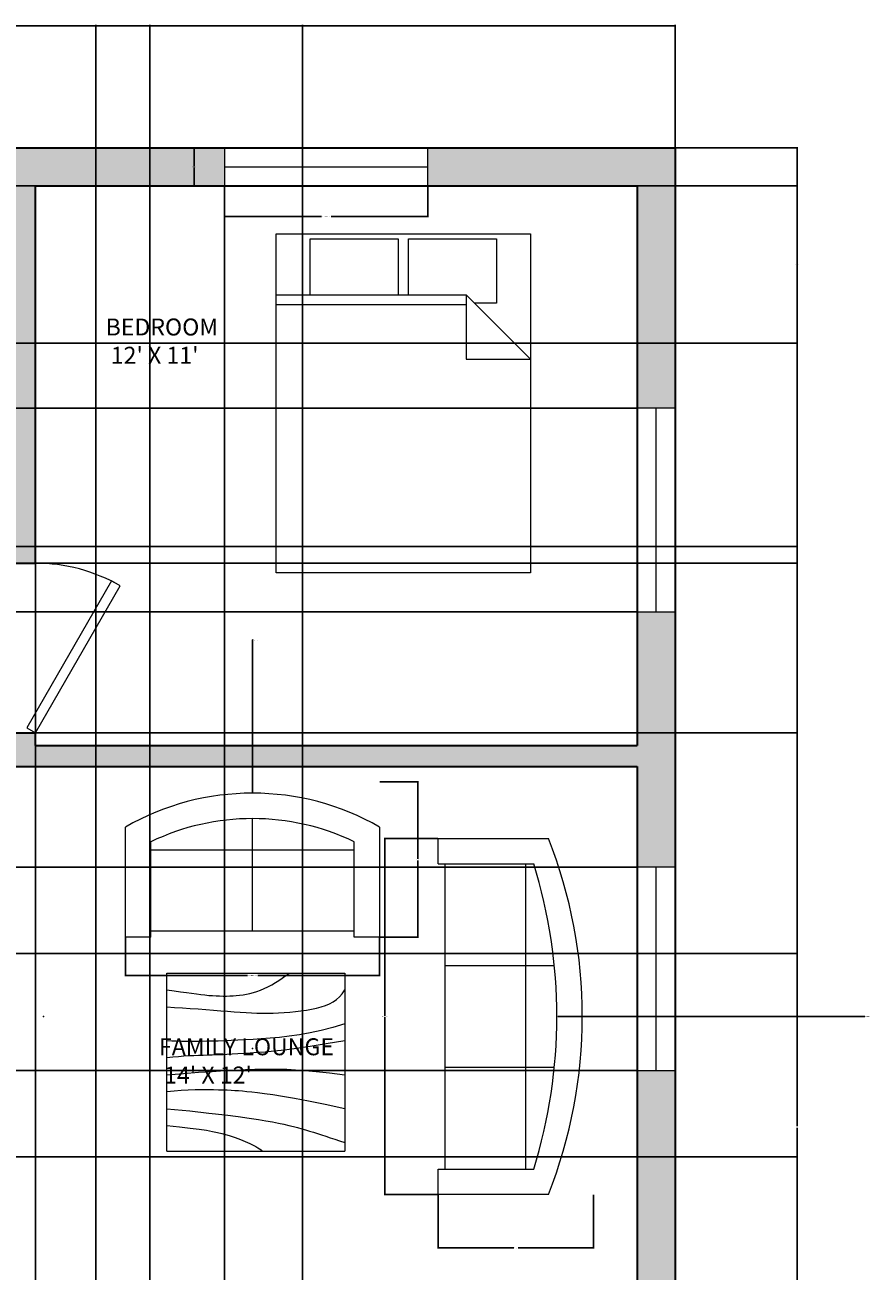
# Model space of a CAD drawing. Units: inches. Extents: x -28 to 649, y -11 to 509.
# Tile 7 of 7: x 450 to 649, y 215 to 509. Entities that reach past the tile are written whole.
import ezdxf

# ---------------------------------------------------------------- set-up
doc = ezdxf.new("R2010")
doc.units = ezdxf.units.IN
doc.header["$MEASUREMENT"] = 0
for name, color, linetype, lineweight in [('A-ANNO-DIMS', 2, 'Continuous', 18), ('A-AREA-IDEN', 18, 'Continuous', 18), ('A-WALL', 7, 'Continuous', 35), ('A-WALL-PATT', 251, 'Continuous', 13), ('doors', 40, 'Continuous', 20), ('furniture', 220, 'Continuous', 18), ('window', 30, 'Continuous', 18)]:
    doc.layers.add(name, color=color, linetype=linetype, lineweight=lineweight)
doc.styles.get("Standard").update_dxf_attribs({"font": 'arial.ttf'})
doc.dimstyles.get("Standard").update_dxf_attribs({"dimtxt": 0.18, "dimasz": 0.18, "dimexe": 0.18, "dimexo": 0.0625, "dimgap": 0.09, "dimtad": 0, "dimtih": 1, "dimtoh": 1, "dimdec": 4, "dimzin": 0, "dimdsep": 46, "dimtxsty": 'Standard', "dimcen": 0.09, "dimadec": 0, "dimazin": 0, "dimtfac": 1, "dimtdec": 4, "dimtofl": 0, "dimtmove": 0, "dimatfit": 3, "dimfxl": 1, "dimtolj": 1, "dimtzin": 0, "dimarcsym": 0})

# ---------------------------------------------------------------- blocks, each defined once
blk = doc.blocks.new('*U10')
for p, q in [((0, 0), (0, 100)), ((750, 0), (750, 100))]:
    blk.add_line(p, q)
blk.add_lwpolyline([(0, 0), (649.5, -375), (671.4, -337.1), (21.9, 37.9)], close=True)
blk.add_arc((0, 0), 750, 330, 0)
blk = doc.blocks.new('Sofa - Roundback 7 ft.')
for p, q in [((-12.00002, -32.4421), (-12.00003, -6.5971)), ((11.99997, -32.4421), (11.99998, -6.5971)), ((-36.000027, -34), (-36.000027, -11.4696)), ((35.99998, -34), (35.99998, -11.4696)), ((-35.999844, -13.3819), (35.9998, -13.3819)), ((-36.000027, -32.4421), (35.99998, -32.4421))]:
    blk.add_line(p, q)
for points in [[(-36.000027, -34), (-42.000027, -34), (-42.000027, -8)], [(41.99998, -8), (41.99998, -34), (35.99998, -34)]]:
    blk.add_lwpolyline(points)
for centre, radius, start, end in [((0, -114.25), 114.25, 68.43141, 111.5686), ((-0.00001, -127.1968), 121.1968, 72.72033, 107.2797)]:
    blk.add_arc(centre, radius, start, end)
blk = doc.blocks.new('Sofa - Roundback Loveseat 5 ft.')
for p, q in [((0, -32.44198), (0, -5.99998)), ((-24, -33.99998), (-24, -11.46958)), ((24.00004, -33.99998), (24.00004, -11.46958)), ((-23.9998, -13.38178), (23.99986, -13.38178)), ((-24, -32.44198), (24.00004, -32.44198))]:
    blk.add_line(p, q)
for points in [[(-24, -33.99998), (-30, -33.99998), (-30, -7.99998)], [(30.00004, -7.99998), (30.00004, -33.99998), (24.00004, -33.99998)]]:
    blk.add_lwpolyline(points)
for centre, radius, start, end in [((0, -60.24998), 60.24998, 60.13715, 119.8628), ((0, -61.38438), 55.38444, 64.32083, 115.6792)]:
    blk.add_arc(centre, radius, start, end)
blk = doc.blocks.new('Bed - Queen')
for p, q in [((0, -80.00003), (0, 0)), ((0, 0), (59.99999, 0)), ((59.99999, 0), (59.99999, -80.00003)), ((7.99999, -1.2), (28.79998, -1.2)), ((7.99999, -14.4), (7.99999, -1.2)), ((28.79998, -1.2), (28.79998, -14.4)), ((31.19999, -1.2), (51.99999, -1.2)), ((31.19999, -14.4), (31.19999, -1.2)), ((51.99999, -1.2), (51.99999, -16.4)), ((0, -14.4), (44.8, -14.4)), ((59.99999, -29.6), (44.8, -14.4)), ((44.8, -14.4), (44.8, -29.6)), ((44.8, -16.8), (0, -16.8)), ((51.99999, -16.4), (46.79936, -16.4)), ((44.8, -29.6), (59.99999, -29.6)), ((59.99999, -80.00003), (0, -80.00003))]:
    blk.add_line(p, q)
blk = doc.blocks.new('Table - Square Woodgrain 42 x 42 in.')
blk.add_line((0, -42), (42, -42))
for points in [[(0, -4), (1.704, -4.2172), (3.2358, -4.4188), (4.615, -4.604), (5.8615, -4.7721), (6.9951, -4.9224), (8.0357, -5.0541), (9.0031, -5.1667), (9.9171, -5.2594), (10.7951, -5.3316), (11.6445, -5.3836), (12.4702, -5.4157), (13.277, -5.4283), (14.0698, -5.4217), (14.8535, -5.3964), (15.6331, -5.3526), (16.4133, -5.2908), (17.1986, -5.2103), (17.9913, -5.1062), (18.793, -4.9727), (19.6056, -4.8038), (20.4307, -4.5937), (21.2701, -4.3365), (22.1256, -4.0262), (22.9989, -3.6571), (23.888, -3.2272), (24.7756, -2.7516), (25.6408, -2.2491), (26.4624, -1.7387), (27.2195, -1.2395), (27.891, -0.7703), (28.456, -0.3501), (28.8934, 0.002)], [(0, -42), (0, 0), (42, 0), (42, -42)], [(0, -8), (1.8203, -8.1001), (3.6741, -8.2149), (5.5411, -8.3408), (7.4011, -8.4741), (9.2339, -8.6112), (11.0193, -8.7484), (12.7371, -8.8821), (14.3671, -9.0086), (15.8954, -9.1246), (17.3337, -9.2278), (18.6997, -9.3159), (20.0116, -9.387), (21.2871, -9.4389), (22.5442, -9.4696), (23.8008, -9.477), (25.0749, -9.459), (26.3791, -9.4137), (27.7049, -9.3403), (29.0383, -9.2382), (30.3655, -9.1068), (31.6728, -8.9455), (32.9461, -8.7535), (34.1717, -8.5304), (35.3358, -8.2756), (36.4268, -7.9863), (37.443, -7.6521), (38.3849, -7.2603), (39.253, -6.7986), (40.048, -6.2542), (40.7705, -5.6147), (41.421, -4.8674), (42, -4)], [(42, -12), (39.1784, -12.8621), (36.4519, -13.5654), (33.8246, -14.1294), (31.3004, -14.5731), (28.8832, -14.9161), (26.577, -15.1775), (24.3858, -15.3768), (22.3136, -15.5332), (20.3622, -15.6632), (18.5254, -15.7718), (16.7947, -15.8612), (15.1618, -15.9338), (13.6183, -15.9916), (12.1558, -16.0369), (10.7659, -16.0718), (9.4403, -16.0987), (8.1703, -16.1191), (6.9461, -16.1325), (5.7577, -16.1377), (4.595, -16.1335), (3.4479, -16.1188), (2.3064, -16.0924), (1.1604, -16.0532), (0, -16)], [(42, -16), (37.6529, -16.7365), (33.8802, -17.329), (30.6179, -17.7961), (27.8015, -18.1561), (25.3668, -18.4275), (23.2497, -18.6288), (21.3859, -18.7785), (19.7111, -18.8949), (18.1693, -18.9939), (16.7375, -19.0795), (15.401, -19.1534), (14.1449, -19.217), (12.9544, -19.2717), (11.8148, -19.3191), (10.7113, -19.3606), (9.6291, -19.3976), (8.5534, -19.4323), (7.47, -19.4689), (6.3643, -19.5122), (5.222, -19.5672), (4.0288, -19.6386), (2.7703, -19.7313), (1.4321, -19.8501), (0, -20)], [(0, -24), (3.9243, -23.6805), (7.4766, -23.4138), (10.6891, -23.1954), (13.5943, -23.0205), (16.2247, -22.8847), (18.6125, -22.7832), (20.7903, -22.7116), (22.7903, -22.6651), (24.6563, -22.642), (26.4764, -22.6507), (28.35, -22.7024), (30.3766, -22.8084), (32.6555, -22.98), (35.2861, -23.2283), (38.3678, -23.5645), (42, -24)], [(42, -32), (37.392, -31.017), (33.4585, -30.2231), (30.1291, -29.5949), (27.3334, -29.109), (25.0009, -28.742), (23.0612, -28.4707), (21.4439, -28.2716), (20.0786, -28.1215), (18.8998, -28.0002), (17.8609, -27.9014), (16.9206, -27.8219), (16.0371, -27.7588), (15.1691, -27.709), (14.2748, -27.6693), (13.3128, -27.6368), (12.2415, -27.6083), (11.0295, -27.5824), (9.6867, -27.5643), (8.233, -27.5608), (6.6884, -27.5787), (5.0728, -27.6248), (3.4062, -27.7058), (1.7086, -27.8286), (0, -28)], [(0, -32), (5.4026, -32.5358), (9.9494, -33.019), (13.7424, -33.4553), (16.8834, -33.8505), (19.4743, -34.2106), (21.6171, -34.5413), (23.4136, -34.8486), (24.9657, -35.1382), (26.3614, -35.4156), (27.6332, -35.6841), (28.7995, -35.9467), (29.8788, -36.2064), (30.8897, -36.4661), (31.8507, -36.7288), (32.7802, -36.9973), (33.6968, -37.2747), (34.6175, -37.5635), (35.5531, -37.8651), (36.5128, -38.1805), (37.506, -38.5108), (38.5421, -38.8568), (39.6302, -39.2197), (40.7797, -39.6004), (42, -40)], [(0, -36), (3.0098, -36.2857), (5.5354, -36.5643), (7.6368, -36.8359), (9.374, -37.1009), (10.807, -37.3597), (11.9957, -37.6126), (13.0002, -37.8599), (13.8804, -38.102), (14.6874, -38.3393), (15.4365, -38.5729), (16.1338, -38.8041), (16.7858, -39.0341), (17.3987, -39.264), (17.9787, -39.4952), (18.5322, -39.7288), (19.0655, -39.9662), (19.5832, -40.2081), (20.0842, -40.4544), (20.5657, -40.7046), (21.0249, -40.9581), (21.459, -41.2144), (21.8653, -41.4731), (22.2409, -41.7335), (22.5831, -41.9951)]]:
    blk.add_lwpolyline(points)
blk = doc.blocks.new('WIN-48x9')
for p, q in [((9, 48), (0, 48)), ((0, 48), (0, 0)), ((4.5, 0), (4.5, 48)), ((9, 0), (9, 48)), ((0, 0), (9, 0)), ((0, 0), (4.5, 0))]:
    blk.add_line(p, q)
blk = doc.blocks.new('*D14')
at = {"layer": 'A-ANNO-DIMS', "color": 0, "lineweight": -2, "transparency": 16777216}
for p, q in [((497.1, 470.88), (497.1, 463.56)), ((545.1, 470.88), (545.1, 463.56)), ((497.28, 463.74), (519.98, 463.74)), ((544.92, 463.74), (522.21, 463.74))]:
    blk.add_line(p, q, dxfattribs=at)
at = {"layer": 'A-ANNO-DIMS', "color": 0, "transparency": 16777216}
for points in [[(497.28, 463.77), (497.28, 463.71), (497.1, 463.74)], [(544.92, 463.77), (544.92, 463.71), (545.1, 463.74)]]:
    blk.add_solid(points, dxfattribs=at)
at = {"layer": 'Defpoints', "color": 0, "transparency": 16777216}
for p in [(497.1, 470.94), (545.1, 470.94), (545.1, 463.74)]:
    blk.add_point(p, dxfattribs=at)
at = {"layer": 'A-ANNO-DIMS', "color": 0, "transparency": 16777216, "insert": (521.1, 463.74), "char_height": 0.18, "attachment_point": 5}
blk.add_mtext('\\A1;WINDOW 48 TYP.', dxfattribs=at)
blk = doc.blocks.new('*D15')
at = {"layer": 'A-ANNO-DIMS', "color": 0, "lineweight": -2, "transparency": 16777216}
for p, q in [((497.03, 479.94), (489.72, 479.94)), ((489.9, 479.76), (489.9, 475.62)), ((489.9, 471.12), (489.9, 475.26)), ((497.03, 470.94), (489.72, 470.94))]:
    blk.add_line(p, q, dxfattribs=at)
at = {"layer": 'A-ANNO-DIMS', "color": 0, "transparency": 16777216}
for points in [[(489.87, 479.76), (489.93, 479.76), (489.9, 479.94)], [(489.87, 471.12), (489.93, 471.12), (489.9, 470.94)]]:
    blk.add_solid(points, dxfattribs=at)
at = {"layer": 'Defpoints', "color": 0, "transparency": 16777216}
for p in [(497.1, 479.94), (489.9, 470.94), (497.1, 470.94)]:
    blk.add_point(p, dxfattribs=at)
at = {"layer": 'A-ANNO-DIMS', "color": 0, "transparency": 16777216, "insert": (489.9, 475.44), "char_height": 0.18, "attachment_point": 5}
blk.add_mtext('\\A1;9 TYP.', dxfattribs=at)
blk = doc.blocks.new('*D24')
at = {"layer": 'A-ANNO-DIMS', "color": 0, "lineweight": -2, "transparency": 16777216}
for p, q in [((547.46, 317.01), (534.75, 317.01)), ((534.93, 316.83), (534.93, 275.19)), ((534.93, 233.19), (534.93, 274.83)), ((547.46, 233.01), (534.75, 233.01))]:
    blk.add_line(p, q, dxfattribs=at)
at = {"layer": 'A-ANNO-DIMS', "color": 0, "transparency": 16777216}
for points in [[(534.9, 316.83), (534.96, 316.83), (534.93, 317.01)], [(534.9, 233.19), (534.96, 233.19), (534.93, 233.01)]]:
    blk.add_solid(points, dxfattribs=at)
at = {"layer": 'Defpoints', "color": 0, "transparency": 16777216}
for p in [(547.53, 317.01), (534.93, 233.01), (547.53, 233.01)]:
    blk.add_point(p, dxfattribs=at)
at = {"layer": 'A-ANNO-DIMS', "color": 0, "transparency": 16777216, "insert": (534.93, 275.01), "char_height": 0.18, "attachment_point": 5}
blk.add_mtext('\\A1;SOFA 84 TYP.', dxfattribs=at)
blk = doc.blocks.new('*D25')
at = {"layer": 'A-ANNO-DIMS', "color": 0, "lineweight": -2, "transparency": 16777216}
for p, q in [((547.53, 232.95), (547.53, 220.23)), ((584.19, 232.95), (584.19, 220.23)), ((547.71, 220.41), (565.33, 220.41)), ((584.01, 220.41), (566.39, 220.41))]:
    blk.add_line(p, q, dxfattribs=at)
at = {"layer": 'A-ANNO-DIMS', "color": 0, "transparency": 16777216}
for points in [[(547.71, 220.44), (547.71, 220.38), (547.53, 220.41)], [(584.01, 220.44), (584.01, 220.38), (584.19, 220.41)]]:
    blk.add_solid(points, dxfattribs=at)
at = {"layer": 'Defpoints', "color": 0, "transparency": 16777216}
for p in [(547.53, 233.01), (584.19, 233.01), (584.19, 220.41)]:
    blk.add_point(p, dxfattribs=at)
at = {"layer": 'A-ANNO-DIMS', "color": 0, "transparency": 16777216, "insert": (565.86, 220.41), "char_height": 0.18, "attachment_point": 5}
blk.add_mtext('\\A1;37 TYP.', dxfattribs=at)
blk = doc.blocks.new('*D26')
at = {"layer": 'A-ANNO-DIMS', "color": 0, "lineweight": -2, "transparency": 16777216}
for p, q in [((473.68, 293.62), (473.68, 284.5)), ((533.68, 293.62), (533.68, 284.5)), ((473.86, 284.68), (502.46, 284.68)), ((533.5, 284.68), (504.9, 284.68))]:
    blk.add_line(p, q, dxfattribs=at)
at = {"layer": 'A-ANNO-DIMS', "color": 0, "transparency": 16777216}
for points in [[(473.86, 284.71), (473.86, 284.65), (473.68, 284.68)], [(533.5, 284.71), (533.5, 284.65), (533.68, 284.68)]]:
    blk.add_solid(points, dxfattribs=at)
at = {"layer": 'Defpoints', "color": 0, "transparency": 16777216}
for p in [(473.68, 293.68), (533.68, 293.68), (533.68, 284.68)]:
    blk.add_point(p, dxfattribs=at)
at = {"layer": 'A-ANNO-DIMS', "color": 0, "transparency": 16777216, "insert": (503.68, 284.68), "char_height": 0.18, "attachment_point": 5}
blk.add_mtext('\\A1;LOVESEAT 60 TYP.', dxfattribs=at)
blk = doc.blocks.new('*D27')
at = {"layer": 'A-ANNO-DIMS', "color": 0, "lineweight": -2, "transparency": 16777216}
for p, q in [((533.74, 330.35), (542.86, 330.35)), ((542.68, 330.17), (542.68, 312.2)), ((542.68, 293.86), (542.68, 311.83)), ((533.74, 293.68), (542.86, 293.68))]:
    blk.add_line(p, q, dxfattribs=at)
at = {"layer": 'A-ANNO-DIMS', "color": 0, "transparency": 16777216}
for points in [[(542.65, 330.17), (542.71, 330.17), (542.68, 330.35)], [(542.65, 293.86), (542.71, 293.86), (542.68, 293.68)]]:
    blk.add_solid(points, dxfattribs=at)
at = {"layer": 'Defpoints', "color": 0, "transparency": 16777216}
for p in [(533.68, 330.35), (542.68, 330.35), (533.68, 293.68)]:
    blk.add_point(p, dxfattribs=at)
at = {"layer": 'A-ANNO-DIMS', "color": 0, "transparency": 16777216, "insert": (542.68, 312.02), "char_height": 0.18, "attachment_point": 5}
blk.add_mtext('\\A1;37 TYP.', dxfattribs=at)
blk = doc.blocks.new('*D30')
at = {"layer": 'A-ANNO-DIMS', "color": 0, "lineweight": -2, "transparency": 16777216}
for p, q in [((27.45, 480), (27.45, 508.92)), ((27.63, 508.74), (315.16, 508.74)), ((603.27, 508.74), (315.74, 508.74)), ((603.45, 480), (603.45, 508.92))]:
    blk.add_line(p, q, dxfattribs=at)
at = {"layer": 'A-ANNO-DIMS', "color": 0, "transparency": 16777216}
for points in [[(27.63, 508.77), (27.63, 508.71), (27.45, 508.74)], [(603.27, 508.77), (603.27, 508.71), (603.45, 508.74)]]:
    blk.add_solid(points, dxfattribs=at)
at = {"layer": 'Defpoints', "color": 0, "transparency": 16777216}
for p in [(603.45, 508.74), (27.45, 479.94), (603.45, 479.94)]:
    blk.add_point(p, dxfattribs=at)
at = {"layer": 'A-ANNO-DIMS', "color": 0, "transparency": 16777216, "insert": (315.45, 508.74), "char_height": 0.18, "attachment_point": 5}
blk.add_mtext('\\A1;576', dxfattribs=at)
blk = doc.blocks.new('*D31')
at = {"layer": 'A-ANNO-DIMS', "color": 0, "lineweight": -2, "transparency": 16777216}
for p, q in [((603.51, 479.94), (632.43, 479.94)), ((632.25, 479.76), (632.25, 249.12)), ((632.25, 18.12), (632.25, 248.76)), ((346.51, 17.94), (632.43, 17.94))]:
    blk.add_line(p, q, dxfattribs=at)
at = {"layer": 'A-ANNO-DIMS', "color": 0, "transparency": 16777216}
for points in [[(632.22, 479.76), (632.28, 479.76), (632.25, 479.94)], [(632.22, 18.12), (632.28, 18.12), (632.25, 17.94)]]:
    blk.add_solid(points, dxfattribs=at)
at = {"layer": 'Defpoints', "color": 0, "transparency": 16777216}
for p in [(603.45, 479.94), (632.25, 479.94), (346.45, 17.94)]:
    blk.add_point(p, dxfattribs=at)
at = {"layer": 'A-ANNO-DIMS', "color": 0, "transparency": 16777216, "insert": (632.25, 248.94), "char_height": 0.18, "attachment_point": 5}
blk.add_mtext('\\A1;462', dxfattribs=at)
blk = doc.blocks.new('*D48')
at = {"layer": 'A-ANNO-DIMS', "color": 0, "lineweight": -2, "transparency": 16777216}
for p, q in [((452.45, 470.88), (452.45, -11.04)), ((497.1, 470.88), (497.1, -11.04)), ((452.63, -10.86), (474.38, -10.86)), ((496.92, -10.86), (475.17, -10.86))]:
    blk.add_line(p, q, dxfattribs=at)
at = {"layer": 'A-ANNO-DIMS', "color": 0, "transparency": 16777216}
for points in [[(452.63, -10.83), (452.63, -10.89), (452.45, -10.86)], [(496.92, -10.83), (496.92, -10.89), (497.1, -10.86)]]:
    blk.add_solid(points, dxfattribs=at)
at = {"layer": 'Defpoints', "color": 0, "transparency": 16777216}
for p in [(452.45, 470.94), (497.1, 470.94), (497.1, -10.86)]:
    blk.add_point(p, dxfattribs=at)
at = {"layer": 'A-ANNO-DIMS', "color": 0, "transparency": 16777216, "insert": (474.77, -10.86), "char_height": 0.18, "attachment_point": 5}
blk.add_mtext('\\A1;44.65', dxfattribs=at)
blk = doc.blocks.new('*D49')
at = {"layer": 'A-ANNO-DIMS', "color": 0, "lineweight": -2, "transparency": 16777216}
for p, q in [((36.51, 470.94), (632.43, 470.94)), ((632.25, 470.76), (632.25, 452.59)), ((632.25, 434.06), (632.25, 452.23)), ((36.51, 433.88), (632.43, 433.88))]:
    blk.add_line(p, q, dxfattribs=at)
at = {"layer": 'A-ANNO-DIMS', "color": 0, "transparency": 16777216}
for points in [[(632.22, 470.76), (632.28, 470.76), (632.25, 470.94)], [(632.22, 434.06), (632.28, 434.06), (632.25, 433.88)]]:
    blk.add_solid(points, dxfattribs=at)
at = {"layer": 'Defpoints', "color": 0, "transparency": 16777216}
for p in [(36.45, 470.94), (36.45, 433.88), (632.25, 433.88)]:
    blk.add_point(p, dxfattribs=at)
at = {"layer": 'A-ANNO-DIMS', "color": 0, "transparency": 16777216, "insert": (632.25, 452.41), "char_height": 0.18, "attachment_point": 5}
blk.add_mtext('\\A1;37.055', dxfattribs=at)
blk = doc.blocks.new('*D50')
at = {"layer": 'A-ANNO-DIMS', "color": 0, "lineweight": -2, "transparency": 16777216}
for p, q in [((594.39, 470.94), (-1.53, 470.94)), ((-1.35, 470.76), (-1.35, 444.89)), ((-1.35, 418.66), (-1.35, 444.53)), ((594.39, 418.48), (-1.53, 418.48))]:
    blk.add_line(p, q, dxfattribs=at)
at = {"layer": 'A-ANNO-DIMS', "color": 0, "transparency": 16777216}
for points in [[(-1.38, 470.76), (-1.32, 470.76), (-1.35, 470.94)], [(-1.38, 418.66), (-1.32, 418.66), (-1.35, 418.48)]]:
    blk.add_solid(points, dxfattribs=at)
at = {"layer": 'Defpoints', "color": 0, "transparency": 16777216}
for p in [(594.45, 470.94), (-1.35, 418.48), (594.45, 418.48)]:
    blk.add_point(p, dxfattribs=at)
at = {"layer": 'A-ANNO-DIMS', "color": 0, "transparency": 16777216, "insert": (-1.35, 444.71), "char_height": 0.18, "attachment_point": 5}
blk.add_mtext('\\A1;52.46', dxfattribs=at)
blk = doc.blocks.new('*D51')
at = {"layer": 'A-ANNO-DIMS', "color": 0, "lineweight": -2, "transparency": 16777216}
for p, q in [((594.39, 370.48), (-1.53, 370.48)), ((-1.35, 370.3), (-1.35, 340.55)), ((-1.35, 310.43), (-1.35, 340.19)), ((594.39, 310.25), (-1.53, 310.25))]:
    blk.add_line(p, q, dxfattribs=at)
at = {"layer": 'A-ANNO-DIMS', "color": 0, "transparency": 16777216}
for points in [[(-1.38, 370.3), (-1.32, 370.3), (-1.35, 370.48)], [(-1.38, 310.43), (-1.32, 310.43), (-1.35, 310.25)]]:
    blk.add_solid(points, dxfattribs=at)
at = {"layer": 'Defpoints', "color": 0, "transparency": 16777216}
for p in [(-1.35, 370.48), (594.45, 370.48), (594.45, 310.25)]:
    blk.add_point(p, dxfattribs=at)
at = {"layer": 'A-ANNO-DIMS', "color": 0, "transparency": 16777216, "insert": (-1.35, 340.37), "char_height": 0.18, "attachment_point": 5}
blk.add_mtext('\\A1;60.23', dxfattribs=at)
blk = doc.blocks.new('*D52')
at = {"layer": 'A-ANNO-DIMS', "color": 0, "lineweight": -2, "transparency": 16777216}
for p, q in [((594.39, 262.25), (-1.53, 262.25)), ((-1.35, 262.07), (-1.35, 206.61)), ((-1.35, 150.79), (-1.35, 206.25)), ((594.39, 150.61), (-1.53, 150.61))]:
    blk.add_line(p, q, dxfattribs=at)
at = {"layer": 'A-ANNO-DIMS', "color": 0, "transparency": 16777216}
for points in [[(-1.38, 262.07), (-1.32, 262.07), (-1.35, 262.25)], [(-1.38, 150.79), (-1.32, 150.79), (-1.35, 150.61)]]:
    blk.add_solid(points, dxfattribs=at)
at = {"layer": 'Defpoints', "color": 0, "transparency": 16777216}
for p in [(-1.35, 262.25), (594.45, 262.25), (594.45, 150.61)]:
    blk.add_point(p, dxfattribs=at)
at = {"layer": 'A-ANNO-DIMS', "color": 0, "transparency": 16777216, "insert": (-1.35, 206.43), "char_height": 0.18, "attachment_point": 5}
blk.add_mtext('\\A1;111.64', dxfattribs=at)
blk = doc.blocks.new('*D53')
at = {"layer": 'A-ANNO-DIMS', "color": 0, "lineweight": -2, "transparency": 16777216}
for p, q in [((36.51, 241.9), (632.43, 241.9)), ((632.25, 241.72), (632.25, 191.76)), ((632.25, 141.44), (632.25, 191.39)), ((36.51, 141.26), (632.43, 141.26))]:
    blk.add_line(p, q, dxfattribs=at)
at = {"layer": 'A-ANNO-DIMS', "color": 0, "transparency": 16777216}
for points in [[(632.22, 241.72), (632.28, 241.72), (632.25, 241.9)], [(632.22, 141.44), (632.28, 141.44), (632.25, 141.26)]]:
    blk.add_solid(points, dxfattribs=at)
at = {"layer": 'Defpoints', "color": 0, "transparency": 16777216}
for p in [(36.45, 241.9), (632.25, 241.9), (36.45, 141.26)]:
    blk.add_point(p, dxfattribs=at)
at = {"layer": 'A-ANNO-DIMS', "color": 0, "transparency": 16777216, "insert": (632.25, 191.58), "char_height": 0.18, "attachment_point": 5}
blk.add_mtext('\\A1;100.64', dxfattribs=at)
blk = doc.blocks.new('*D54')
at = {"layer": 'A-ANNO-DIMS', "color": 0, "lineweight": -2, "transparency": 16777216}
for p, q in [((36.51, 385.88), (632.43, 385.88)), ((632.25, 385.7), (632.25, 338.07)), ((632.25, 290.08), (632.25, 337.71)), ((36.51, 289.9), (632.43, 289.9))]:
    blk.add_line(p, q, dxfattribs=at)
at = {"layer": 'A-ANNO-DIMS', "color": 0, "transparency": 16777216}
for points in [[(632.22, 385.7), (632.28, 385.7), (632.25, 385.88)], [(632.22, 290.08), (632.28, 290.08), (632.25, 289.9)]]:
    blk.add_solid(points, dxfattribs=at)
at = {"layer": 'Defpoints', "color": 0, "transparency": 16777216}
for p in [(36.45, 385.88), (632.25, 385.88), (36.45, 289.9)]:
    blk.add_point(p, dxfattribs=at)
at = {"layer": 'A-ANNO-DIMS', "color": 0, "transparency": 16777216, "insert": (632.25, 337.89), "char_height": 0.18, "attachment_point": 5}
blk.add_mtext('\\A1;95.99', dxfattribs=at)
blk = doc.blocks.new('*D60')
at = {"layer": 'A-ANNO-DIMS', "color": 0, "lineweight": -2, "transparency": 16777216}
for p, q in [((479.45, 206), (479.45, 508.92)), ((479.63, 508.74), (497.23, 508.74)), ((515.27, 508.74), (497.67, 508.74)), ((515.45, 206), (515.45, 508.92))]:
    blk.add_line(p, q, dxfattribs=at)
at = {"layer": 'A-ANNO-DIMS', "color": 0, "transparency": 16777216}
for points in [[(479.63, 508.77), (479.63, 508.71), (479.45, 508.74)], [(515.27, 508.77), (515.27, 508.71), (515.45, 508.74)]]:
    blk.add_solid(points, dxfattribs=at)
at = {"layer": 'Defpoints', "color": 0, "transparency": 16777216}
for p in [(515.45, 508.74), (479.45, 205.94), (515.45, 205.94)]:
    blk.add_point(p, dxfattribs=at)
at = {"layer": 'A-ANNO-DIMS', "color": 0, "transparency": 16777216, "insert": (497.45, 508.74), "char_height": 0.18, "attachment_point": 5}
blk.add_mtext('\\A1;36', dxfattribs=at)
blk = doc.blocks.new('*D65')
at = {"layer": 'A-ANNO-DIMS', "color": 0, "lineweight": -2, "transparency": 16777216}
for p, q in [((185.51, 381.94), (632.43, 381.94)), ((632.25, 381.76), (632.25, 362.12)), ((632.25, 342.12), (632.25, 361.76)), ((185.51, 341.94), (632.43, 341.94))]:
    blk.add_line(p, q, dxfattribs=at)
at = {"layer": 'A-ANNO-DIMS', "color": 0, "transparency": 16777216}
for points in [[(632.22, 381.76), (632.28, 381.76), (632.25, 381.94)], [(632.22, 342.12), (632.28, 342.12), (632.25, 341.94)]]:
    blk.add_solid(points, dxfattribs=at)
at = {"layer": 'Defpoints', "color": 0, "transparency": 16777216}
for p in [(185.45, 381.94), (632.25, 381.94), (185.45, 341.94)]:
    blk.add_point(p, dxfattribs=at)
at = {"layer": 'A-ANNO-DIMS', "color": 0, "transparency": 16777216, "insert": (632.25, 361.94), "char_height": 0.18, "attachment_point": 5}
blk.add_mtext('\\A1;40', dxfattribs=at)
blk = doc.blocks.new('*D68')
at = {"layer": 'A-ANNO-DIMS', "color": 0, "lineweight": -2, "transparency": 16777216}
for p, q in [((358.05, 91.23), (358.05, 508.92)), ((358.23, 508.74), (411.94, 508.74)), ((466.55, 508.74), (412.85, 508.74)), ((466.73, 91.23), (466.73, 508.92))]:
    blk.add_line(p, q, dxfattribs=at)
at = {"layer": 'A-ANNO-DIMS', "color": 0, "transparency": 16777216}
for points in [[(358.23, 508.77), (358.23, 508.71), (358.05, 508.74)], [(466.55, 508.77), (466.55, 508.71), (466.73, 508.74)]]:
    blk.add_solid(points, dxfattribs=at)
at = {"layer": 'Defpoints', "color": 0, "transparency": 16777216}
for p in [(466.73, 508.74), (358.05, 91.17), (466.73, 91.17)]:
    blk.add_point(p, dxfattribs=at)
at = {"layer": 'A-ANNO-DIMS', "color": 0, "transparency": 16777216, "insert": (412.39, 508.74), "char_height": 0.18, "attachment_point": 5}
blk.add_mtext('\\A1;108.68', dxfattribs=at)
blk = doc.blocks.new('*D77')
at = {"layer": 'A-ANNO-DIMS', "color": 0, "lineweight": -2, "transparency": 16777216}
for p, q in [((454.24, 275.01), (454.42, 275.01)), ((454.33, 274.92), (454.33, 275.1)), ((648.25, 275.01), (575.71, 275.01))]:
    blk.add_line(p, q, dxfattribs=at)
at = {"layer": 'A-ANNO-DIMS', "color": 0, "transparency": 16777216}
blk.add_solid([(575.71, 275.04), (575.71, 274.98), (575.53, 275.01)], dxfattribs=at)
at = {"layer": 'Defpoints', "color": 0, "transparency": 16777216}
for p in [(454.33, 275.01), (575.53, 275.01)]:
    blk.add_point(p, dxfattribs=at)
at = {"layer": 'A-ANNO-DIMS', "color": 0, "transparency": 16777216, "insert": (648.92, 275.01), "char_height": 0.18, "attachment_point": 5}
blk.add_mtext('\\A1;2X R121.2', dxfattribs=at)
blk = doc.blocks.new('*D79')
at = {"layer": 'A-ANNO-DIMS', "color": 0, "lineweight": -2, "transparency": 16777216}
for p, q in [((503.86, 363.83), (503.68, 363.83)), ((503.68, 363.83), (503.68, 327.86)), ((503.68, 267.34), (503.68, 267.52)), ((503.59, 267.43), (503.77, 267.43))]:
    blk.add_line(p, q, dxfattribs=at)
at = {"layer": 'A-ANNO-DIMS', "color": 0, "transparency": 16777216}
blk.add_solid([(503.65, 327.86), (503.71, 327.86), (503.68, 327.68)], dxfattribs=at)
at = {"layer": 'Defpoints', "color": 0, "transparency": 16777216}
for p in [(503.68, 327.68), (503.68, 267.43)]:
    blk.add_point(p, dxfattribs=at)
at = {"layer": 'A-ANNO-DIMS', "color": 0, "transparency": 16777216, "insert": (504.53, 363.83), "char_height": 0.18, "attachment_point": 5}
blk.add_mtext('\\A1;2X R60.25', dxfattribs=at)

msp = doc.modelspace()

# ---------------------------------------------------------------- hatches: boundary and pattern name
at = {"layer": 'A-WALL-PATT'}
h = msp.add_hatch(color=256, dxfattribs=at)
h.dxf.hatch_style = 1
h.paths.add_polyline_path([(36.4499, 184.9382), (165.4499, 184.9382), (165.4499, 189.9382), (36.4499, 189.9382), (36.4499, 241.898), (27.4499, 241.898), (27.4499, 141.2558), (36.4499, 141.2558)])
h.paths.add_polyline_path([(36.4499, 385.8835), (27.4499, 385.8835), (27.4499, 289.898), (36.4499, 289.898)])
h.paths.add_polyline_path([(185.4499, 341.9382), (180.4499, 341.9382), (180.4499, 338.9382), (36.4499, 338.9382), (36.4499, 333.9382), (185.4499, 333.9382)])
h.paths.add_polyline_path([(36.4499, 470.9382), (79.2168, 470.9382), (79.2168, 479.9382), (27.4499, 479.9382), (27.4499, 433.8835), (36.4499, 433.8835)])
h.paths.add_polyline_path([(185.4499, 470.9382), (203.9104, 470.9382), (203.9104, 479.9382), (127.2168, 479.9382), (127.2168, 470.9382), (180.4499, 470.9382), (180.4499, 381.9382), (188.4499, 381.9382), (188.4499, 386.9382), (185.4499, 386.9382)])
h.paths.add_polyline_path([(292.4601, 479.9382), (227.9104, 479.9382), (227.9104, 470.9382), (245.4499, 470.9382), (245.4499, 386.9382), (217.4499, 386.9382), (217.4499, 381.9382), (245.4499, 381.9382), (245.4499, 338.9382), (245.4499, 333.9382), (251.5222, 333.9382), (251.5222, 338.9382), (250.4499, 338.9382), (250.4499, 470.9382), (292.4601, 470.9382)])
h.paths.add_polyline_path([(410.9121, 479.9382), (340.4601, 479.9382), (340.4601, 470.9382), (382.4499, 470.9382), (382.4499, 338.9382), (287.5222, 338.9382), (287.5222, 333.9382), (387.4499, 333.9382), (387.4499, 381.9382), (415.4499, 381.9382), (415.4499, 386.9382), (387.4499, 386.9382), (387.4499, 470.9382), (410.9121, 470.9382)])
h.paths.add_polyline_path([(497.0961, 479.9382), (434.9121, 479.9382), (434.9121, 470.9382), (447.4499, 470.9382), (447.4499, 386.9382), (444.4499, 386.9382), (444.4499, 381.9382), (452.4499, 381.9382), (452.4499, 470.9382), (497.0961, 470.9382)])
h.paths.add_polyline_path([(603.4499, 479.9382), (545.0961, 479.9382), (545.0961, 470.9382), (594.4499, 470.9382), (594.4499, 418.4819), (603.4499, 418.4819)])
h.paths.add_polyline_path([(603.4499, 370.4819), (594.4499, 370.4819), (594.4499, 338.9382), (452.4499, 338.9382), (452.4499, 341.9382), (447.4499, 341.9382), (447.4499, 338.9382), (447.4499, 333.9382), (594.4499, 333.9382), (594.4499, 310.2528), (603.4499, 310.2528)])
h.paths.add_polyline_path([(603.4499, 262.2528), (594.4499, 262.2528), (594.4499, 205.9382), (515.4499, 205.9382), (515.4499, 200.9382), (594.4499, 200.9382), (594.4499, 150.6102), (603.4499, 150.6102)])

# ---------------------------------------------------------------- linework, layer by layer
at = {"layer": 'A-WALL'}
for p, q in [((452.4499, 470.9382), (594.4499, 470.9382)), ((452.4499, 381.9382), (452.4499, 470.9382)), ((594.4499, 470.9382), (594.4499, 338.9382)), ((444.4499, 381.9382), (452.4499, 381.9382)), ((447.4499, 341.9382), (452.4499, 341.9382)), ((452.4499, 338.9382), (452.4499, 341.9382)), ((452.4499, 338.9382), (594.4499, 338.9382)), ((447.4499, 333.9382), (594.4499, 333.9382)), ((594.4499, 333.9382), (594.4499, 205.9382))]:
    msp.add_line(p, q, dxfattribs=at)
msp.add_lwpolyline([(209.4499, 47.9382), (27.4499, 47.9382), (27.4499, 479.9382), (603.4499, 479.9382), (603.4499, 47.9382), (269.4499, 47.9382)], dxfattribs=at)

# ---------------------------------------------------------------- block references
at = {"layer": 'doors', "xscale": 0.0533333333333356, "yscale": 0.0533333333333356, "zscale": 0.0533333333333356, "rotation": 90}
msp.add_blockref('*U10', (452.4499, 341.9382), dxfattribs=at)
at = {"layer": 'furniture'}
for name, p in [('Bed - Queen', (509.285, 459.6524)), ('Sofa - Roundback Loveseat 5 ft.', (503.679, 327.6832)), ('Table - Square Woodgrain 42 x 42 in.', (483.444, 285.2521))]:
    msp.add_blockref(name, p, dxfattribs=at)
at = {"layer": 'furniture', "rotation": 270}
msp.add_blockref('Sofa - Roundback 7 ft.', (581.5274, 275.0109), dxfattribs=at)
at = {"layer": 'window', "rotation": 269.999999999989}
msp.add_blockref('WIN-48x9', (497.0961, 479.9382), dxfattribs=at)
at = {"layer": 'window'}
for p in [(594.4499, 370.4819), (594.4499, 262.2528)]:
    msp.add_blockref('WIN-48x9', p, dxfattribs=at)

# ---------------------------------------------------------------- texts
at = {"layer": 'A-AREA-IDEN', "char_height": 4, "attachment_point": 1}
for s, insert in [("BEDROOM\\P 12' X 11'", (469.0022, 439.6565)), ("FAMILY LOUNGE\\P 14' X 12'", (481.6022, 269.8571))]:
    msp.add_mtext_dynamic_manual_height_columns(s, width=46.696275, gutter_width=1, heights=[0], dxfattribs=dict(at, insert=insert))

# ---------------------------------------------------------------- dimensions: what is measured, and where the dimension line sits
at = {"layer": 'A-ANNO-DIMS'}
for base, p1, p2, override, picture, middle in [((603.4499, 508.7392), (27.4499, 479.9382), (603.4499, 479.9382), {"dimdec": 0, "dimlfac": 1, "dimrnd": 0, "dimzin": 0, "dimdsep": 46, "dimlunit": 2}, '*D30', (315.4499, 508.7392)), ((466.7314, 508.7392), (358.0522, 91.1694), (466.7314, 91.1694), {"dimdec": 2, "dimlfac": 1, "dimrnd": 0, "dimzin": 0, "dimdsep": 46, "dimlunit": 2}, '*D68', (412.3918, 508.7392)), ((515.4499, 508.7392), (479.4499, 205.9382), (515.4499, 205.9382), {"dimdec": 0, "dimlfac": 1, "dimrnd": 0, "dimzin": 0, "dimdsep": 46, "dimlunit": 2}, '*D60', (497.4499, 508.7392)), ((497.0961, -10.8628), (452.4499, 470.9382), (497.0961, 470.9382), {"dimdec": 2, "dimlfac": 1, "dimrnd": 0, "dimzin": 0, "dimdsep": 46, "dimlunit": 2}, '*D48', (474.773, -10.8628))]:
    dim = msp.add_linear_dim(base=base, p1=p1, p2=p2, dimstyle='Standard', override=override, dxfattribs=at)
    dim.commit()
    dim.dimension.update_dxf_attribs({"geometry": picture, "text_midpoint": middle})
for base, p1, p2, override, picture, middle in [((632.2509, 479.9382), (346.4499, 17.9382), (603.4499, 479.9382), {"dimdec": 0, "dimlfac": 1, "dimrnd": 0, "dimzin": 0, "dimdsep": 46, "dimlunit": 2}, '*D31', (632.2509, 248.9382)), ((-1.3511, 418.4819), (594.4499, 470.9382), (594.4499, 418.4819), {"dimdec": 2, "dimlfac": 1, "dimrnd": 0, "dimzin": 0, "dimdsep": 46, "dimlunit": 2}, '*D50', (-1.3511, 444.71)), ((632.2509, 433.8835), (36.4499, 470.9382), (36.4499, 433.8835), {"dimdec": 3, "dimlfac": 1, "dimrnd": 0, "dimzin": 0, "dimdsep": 46, "dimlunit": 2}, '*D49', (632.2509, 452.4109)), ((632.2509, 385.8835), (36.4499, 289.898), (36.4499, 385.8835), {"dimdec": 2, "dimlfac": 1, "dimrnd": 0, "dimzin": 0, "dimdsep": 46, "dimlunit": 2}, '*D54', (632.2509, 337.8907)), ((632.2509, 381.9382), (185.4499, 341.9382), (185.4499, 381.9382), {"dimdec": 0, "dimlfac": 1, "dimrnd": 0, "dimzin": 0, "dimdsep": 46, "dimlunit": 2}, '*D65', (632.2509, 361.9382)), ((-1.3511, 370.4819), (594.4499, 310.2528), (594.4499, 370.4819), {"dimdec": 2, "dimlfac": 1, "dimrnd": 0, "dimzin": 0, "dimdsep": 46, "dimlunit": 2}, '*D51', (-1.3511, 340.3674)), ((-1.3511, 262.2528), (594.4499, 150.6102), (594.4499, 262.2528), {"dimdec": 2, "dimlfac": 1, "dimrnd": 0, "dimzin": 0, "dimdsep": 46, "dimlunit": 2}, '*D52', (-1.3511, 206.4315)), ((632.2509, 241.898), (36.4499, 141.2558), (36.4499, 241.898), {"dimdec": 2, "dimlfac": 1, "dimrnd": 0, "dimzin": 0, "dimdsep": 46, "dimlunit": 2}, '*D53', (632.2509, 191.5769))]:
    dim = msp.add_linear_dim(base=base, p1=p1, p2=p2, angle=90, dimstyle='Standard', override=override, dxfattribs=at)
    dim.commit()
    dim.dimension.update_dxf_attribs({"geometry": picture, "text_midpoint": middle})
for base, p1, p2, angle, text, picture, middle in [((489.8961, 470.9382), (497.0961, 479.9382), (497.0961, 470.9382), 270, '<> TYP.', '*D15', (489.8961, 475.4382)), ((542.679, 330.3499), (533.679, 293.6832), (533.679, 330.3499), 90, '<> TYP.', '*D27', (542.679, 312.0165)), ((534.9274, 233.0109), (547.5274, 317.0109), (547.5274, 233.0109), 270, 'SOFA <> TYP.', '*D24', (534.9274, 275.0109))]:
    dim = msp.add_linear_dim(base=base, p1=p1, p2=p2, angle=angle, text=text, dimstyle='Standard', override={"dimdec": 0, "dimlfac": 1, "dimrnd": 0, "dimzin": 0, "dimdsep": 46, "dimlunit": 2}, dxfattribs=at)
    dim.commit()
    dim.dimension.update_dxf_attribs({"geometry": picture, "text_midpoint": middle})
for base, p1, p2, text, picture, middle in [((545.0961, 463.7382), (497.0961, 470.9382), (545.0961, 470.9382), 'WINDOW <> TYP.', '*D14', (521.0961, 463.7382)), ((533.679, 284.6832), (473.679, 293.6832), (533.679, 293.6832), 'LOVESEAT <> TYP.', '*D26', (503.679, 284.6832)), ((584.194, 220.4109), (547.5274, 233.0109), (584.194, 233.0109), '<> TYP.', '*D25', (565.8607, 220.4109))]:
    dim = msp.add_linear_dim(base=base, p1=p1, p2=p2, text=text, dimstyle='Standard', override={"dimdec": 0, "dimlfac": 1, "dimrnd": 0, "dimzin": 0, "dimdsep": 46, "dimlunit": 2}, dxfattribs=at)
    dim.commit()
    dim.dimension.update_dxf_attribs({"geometry": picture, "text_midpoint": middle})
for center, mpoint, override, picture, middle in [((503.679, 267.4332), (503.679, 327.6832), {"dimdec": 2, "dimlfac": 1, "dimrnd": 0, "dimzin": 0, "dimdsep": 46, "dimlunit": 2}, '*D79', (504.5344, 363.8332)), ((454.3306, 275.0109), (575.5274, 275.011), {"dimdec": 1, "dimlfac": 1, "dimrnd": 0, "dimzin": 0, "dimdsep": 46, "dimlunit": 2}, '*D77', (648.2455, 275.011))]:
    dim = msp.add_radius_dim(center=center, mpoint=mpoint, text='2X <>', dimstyle='Standard', override=override, dxfattribs=at)
    dim.commit()
    dim.dimension.update_dxf_attribs({"geometry": picture, "text_midpoint": middle, "dimtype": 164})

doc.saveas('drawing.dxf')
